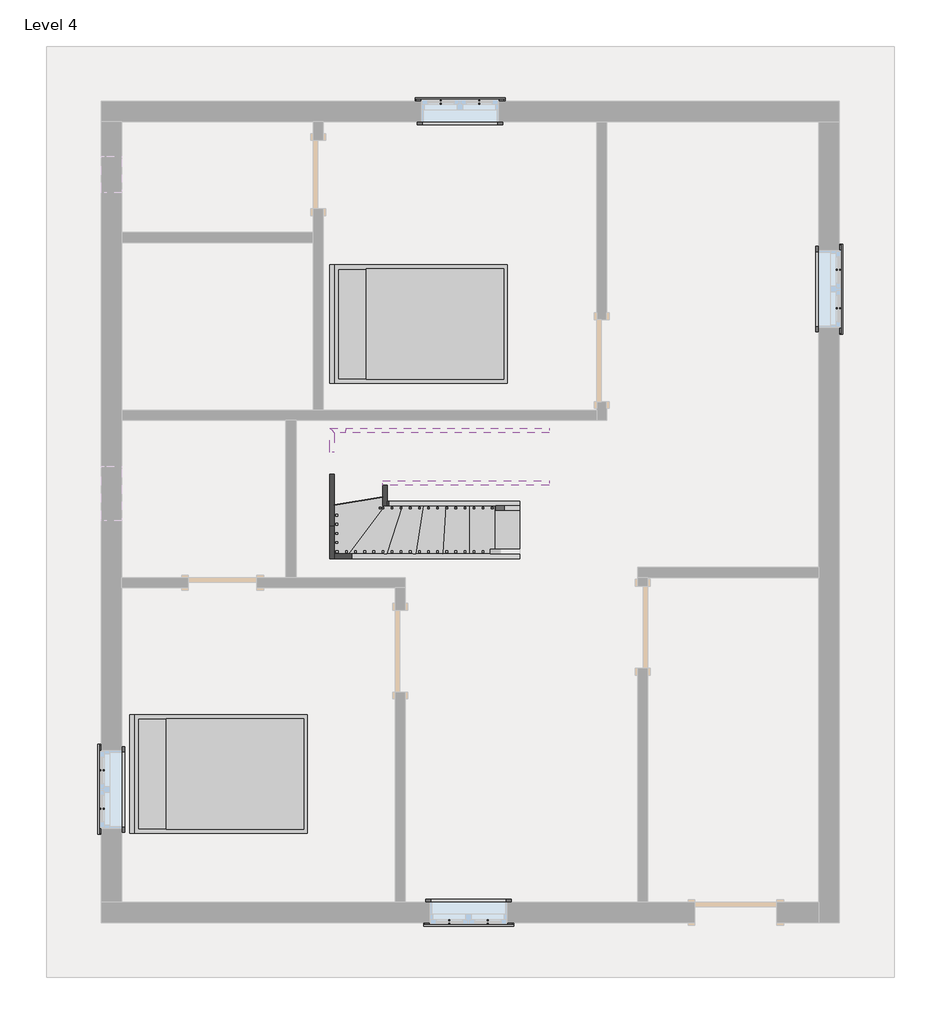
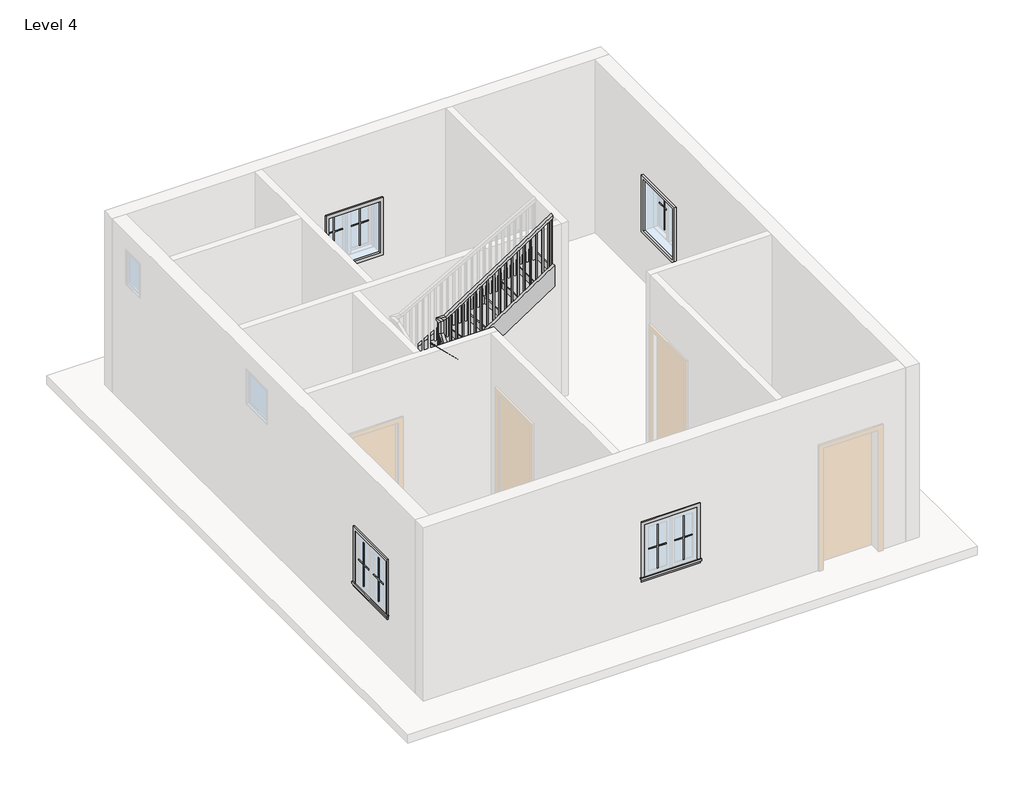
# One storey, part 2 of 2: 16 proxies, 9 members, 2 furniture elements, 1 railing, 1 stair flight.
"""IFC4 building model written with IfcOpenShell, lengths in millimetres."""

from ifc_helpers import new_model, si_unit, frame, origin, place, context, project, spatial, polyline, outline, extrude, faceted_brep, transform, mapped, element, save
from components import muntin_pattern_2x2_muntin_pattern_2x2_b3fe6957, muntin_pattern_2x2_muntin_pattern_2x2_3e0ecaf2, trim_window_exterior_flat_with_sill_41619996, trim_window_interior_flat_picture_frame_51c85655, bed_17739_bed_17739_15c61121, stair_flight_033e9654

model = new_model("IFC4")

# Units and contexts
model_context = context("Model", 3, world=origin())
ifc_project = project(units=[si_unit("LENGTHUNIT", "METRE", prefix="MILLI")], contexts=[model_context])

# Site, building, storey
site = spatial("IfcSite", under=ifc_project)
building = spatial("IfcBuilding", under=site)
storey = spatial("IfcBuildingStorey", under=building, Name="Level 4", Elevation=6400.8)

# Proxies
placement = place(None, origin())
muntin_pattern_2x2_muntin_pattern_2x2_shape = muntin_pattern_2x2_muntin_pattern_2x2_b3fe6957(model_context)
element("IfcBuildingElementProxy", 1, Name="Muntin Pattern_2x2 : Muntin Pattern_2x2", ObjectType="Muntin Pattern_2x2 : Muntin Pattern_2x2", at=placement, inside=storey, context=model_context, shape_type="MappedRepresentation", body=[
    mapped(muntin_pattern_2x2_muntin_pattern_2x2_shape, transform((-1143.3273498, 4766.5933073, 7385.05), x_axis=(1.0, 0.0, 0.0), y_axis=(0.0, 1.0, 0.0), z_axis=(0.0, 0.0, 1.0))),
])
element("IfcBuildingElementProxy", 2, Name="Muntin Pattern_2x2 : Muntin Pattern_2x2", ObjectType="Muntin Pattern_2x2 : Muntin Pattern_2x2", at=placement, inside=storey, context=model_context, shape_type="MappedRepresentation", body=[
    mapped(muntin_pattern_2x2_muntin_pattern_2x2_shape, transform((3290.5601502, 2894.9308073, 7385.05), x_axis=(0.0, -1.0, 0.0), y_axis=(1.0, 0.0, 0.0), z_axis=(0.0, 0.0, 1.0))),
])
element("IfcBuildingElementProxy", 3, Name="Muntin Pattern_2x2 : Muntin Pattern_2x2", ObjectType="Muntin Pattern_2x2 : Muntin Pattern_2x2", at=placement, inside=storey, context=model_context, shape_type="MappedRepresentation", body=[
    mapped(muntin_pattern_2x2_muntin_pattern_2x2_shape, transform((-619.4523498, -4374.2316927, 7385.05), x_axis=(-1.0, 0.0, 0.0), y_axis=(0.0, -1.0, 0.0), z_axis=(0.0, 0.0, 1.0))),
])
element("IfcBuildingElementProxy", 4, Name="Muntin Pattern_2x2 : Muntin Pattern_2x2", ObjectType="Muntin Pattern_2x2 : Muntin Pattern_2x2", at=placement, inside=storey, context=model_context, shape_type="MappedRepresentation", body=[
    mapped(muntin_pattern_2x2_muntin_pattern_2x2_shape, transform((-4919.9898498, -3112.1691927, 7385.05), x_axis=(0.0, 1.0, 0.0), y_axis=(-1.0, 0.0, 0.0), z_axis=(0.0, 0.0, 1.0))),
])
muntin_pattern_2x2_muntin_pattern_2x2_2_shape = muntin_pattern_2x2_muntin_pattern_2x2_3e0ecaf2(model_context)
element("IfcBuildingElementProxy", 5, Name="Muntin Pattern_2x2 : Muntin Pattern_2x2", ObjectType="Muntin Pattern_2x2 : Muntin Pattern_2x2", at=placement, inside=storey, context=model_context, shape_type="MappedRepresentation", body=[
    mapped(muntin_pattern_2x2_muntin_pattern_2x2_2_shape, transform((-714.7023498, 4766.5933073, 7385.05), x_axis=(-1.0, 0.0, 0.0), y_axis=(0.0, -1.0, 0.0), z_axis=(0.0, 0.0, 1.0))),
])
element("IfcBuildingElementProxy", 6, Name="Muntin Pattern_2x2 : Muntin Pattern_2x2", ObjectType="Muntin Pattern_2x2 : Muntin Pattern_2x2", at=placement, inside=storey, context=model_context, shape_type="MappedRepresentation", body=[
    mapped(muntin_pattern_2x2_muntin_pattern_2x2_2_shape, transform((3290.5601502, 2466.3058073, 7385.05), x_axis=(0.0, 1.0, 0.0), y_axis=(-1.0, 0.0, 0.0), z_axis=(0.0, 0.0, 1.0))),
])
element("IfcBuildingElementProxy", 7, Name="Muntin Pattern_2x2 : Muntin Pattern_2x2", ObjectType="Muntin Pattern_2x2 : Muntin Pattern_2x2", at=placement, inside=storey, context=model_context, shape_type="MappedRepresentation", body=[
    mapped(muntin_pattern_2x2_muntin_pattern_2x2_2_shape, transform((-1048.0773498, -4374.2316927, 7385.05), x_axis=(1.0, 0.0, 0.0), y_axis=(0.0, 1.0, 0.0), z_axis=(0.0, 0.0, 1.0))),
])
element("IfcBuildingElementProxy", 8, Name="Muntin Pattern_2x2 : Muntin Pattern_2x2", ObjectType="Muntin Pattern_2x2 : Muntin Pattern_2x2", at=placement, inside=storey, context=model_context, shape_type="MappedRepresentation", body=[
    mapped(muntin_pattern_2x2_muntin_pattern_2x2_2_shape, transform((-4919.9898498, -2683.5441927, 7385.05), x_axis=(0.0, -1.0, 0.0), y_axis=(1.0, 0.0, 0.0), z_axis=(0.0, 0.0, 1.0))),
])
trim_window_exterior_flat_with_sill_shape = trim_window_exterior_flat_with_sill_41619996(model_context)
element("IfcBuildingElementProxy", 9, Name="Trim-Window-Exterior-Flat : with Sill", ObjectType="Trim-Window-Exterior-Flat : with Sill", at=placement, inside=storey, context=model_context, shape_type="MappedRepresentation", body=[
    mapped(trim_window_exterior_flat_with_sill_shape, transform((-929.0148498, 4776.1183073, 8229.6), x_axis=(-1.0, 0.0, 0.0), y_axis=(0.0, 0.0, 1.0), z_axis=(0.0, 1.0, 0.0))),
])
element("IfcBuildingElementProxy", 10, Name="Trim-Window-Exterior-Flat : with Sill", ObjectType="Trim-Window-Exterior-Flat : with Sill", at=placement, inside=storey, context=model_context, shape_type="MappedRepresentation", body=[
    mapped(trim_window_exterior_flat_with_sill_shape, transform((3300.0851502, 2680.6183073, 8229.6), x_axis=(0.0, 1.0, 0.0), y_axis=(0.0, 0.0, 1.0), z_axis=(1.0, 0.0, 0.0))),
])
element("IfcBuildingElementProxy", 11, Name="Trim-Window-Exterior-Flat : with Sill", ObjectType="Trim-Window-Exterior-Flat : with Sill", at=placement, inside=storey, context=model_context, shape_type="MappedRepresentation", body=[
    mapped(trim_window_exterior_flat_with_sill_shape, transform((-833.7648498, -4383.7566927, 8229.6), x_axis=(1.0, 0.0, 0.0), y_axis=(0.0, 0.0, 1.0), z_axis=(0.0, -1.0, 0.0))),
])
element("IfcBuildingElementProxy", 12, Name="Trim-Window-Exterior-Flat : with Sill", ObjectType="Trim-Window-Exterior-Flat : with Sill", at=placement, inside=storey, context=model_context, shape_type="MappedRepresentation", body=[
    mapped(trim_window_exterior_flat_with_sill_shape, transform((-4929.5148498, -2897.8566927, 8229.6), x_axis=(0.0, -1.0, 0.0), y_axis=(0.0, 0.0, 1.0), z_axis=(-1.0, 0.0, 0.0))),
])
trim_window_interior_flat_picture_frame_shape = trim_window_interior_flat_picture_frame_51c85655(model_context)
element("IfcBuildingElementProxy", 13, Name="Trim-Window-Interior-Flat : Picture Frame", ObjectType="Trim-Window-Interior-Flat : Picture Frame", at=placement, inside=storey, context=model_context, shape_type="MappedRepresentation", body=[
    mapped(trim_window_interior_flat_picture_frame_shape, transform((-929.0148498, 4547.5183073, 8229.6), x_axis=(1.0, 0.0, 0.0), y_axis=(0.0, 0.0, 1.0), z_axis=(0.0, -1.0, 0.0))),
])
element("IfcBuildingElementProxy", 14, Name="Trim-Window-Interior-Flat : Picture Frame", ObjectType="Trim-Window-Interior-Flat : Picture Frame", at=placement, inside=storey, context=model_context, shape_type="MappedRepresentation", body=[
    mapped(trim_window_interior_flat_picture_frame_shape, transform((3071.4851502, 2680.6183073, 8229.6), x_axis=(0.0, -1.0, 0.0), y_axis=(0.0, 0.0, 1.0), z_axis=(-1.0, 0.0, 0.0))),
])
element("IfcBuildingElementProxy", 15, Name="Trim-Window-Interior-Flat : Picture Frame", ObjectType="Trim-Window-Interior-Flat : Picture Frame", at=placement, inside=storey, context=model_context, shape_type="MappedRepresentation", body=[
    mapped(trim_window_interior_flat_picture_frame_shape, transform((-833.7648498, -4155.1566927, 8229.6), x_axis=(-1.0, 0.0, 0.0), y_axis=(0.0, 0.0, 1.0), z_axis=(0.0, 1.0, 0.0))),
])
element("IfcBuildingElementProxy", 16, Name="Trim-Window-Interior-Flat : Picture Frame", ObjectType="Trim-Window-Interior-Flat : Picture Frame", at=placement, inside=storey, context=model_context, shape_type="MappedRepresentation", body=[
    mapped(trim_window_interior_flat_picture_frame_shape, transform((-4700.9148498, -2897.8566927, 8229.6), x_axis=(0.0, 1.0, 0.0), y_axis=(0.0, 0.0, 1.0), z_axis=(1.0, 0.0, 0.0))),
])

# Furniture
bed_17739_bed_17739_shape = bed_17739_bed_17739_15c61121(model_context)
element("IfcFurniture", 17, ObjectType="Bed_17739 : Bed_17739", at=placement, inside=storey, context=model_context, shape_type="MappedRepresentation", body=[
    mapped(bed_17739_bed_17739_shape, transform((-3596.0148498, -2726.4066927, 6400.8), x_axis=(0.0, 1.0, 0.0), y_axis=(-1.0, 0.0, 0.0), z_axis=(0.0, 0.0, 1.0))),
])
element("IfcFurniture", 18, ObjectType="Bed_17739 : Bed_17739", at=placement, inside=storey, context=model_context, shape_type="MappedRepresentation", body=[
    mapped(bed_17739_bed_17739_shape, transform((-1367.1648498, 2290.0933073, 6400.8), x_axis=(0.0, 1.0, 0.0), y_axis=(-1.0, 0.0, 0.0), z_axis=(0.0, 0.0, 1.0))),
])

# Members
element("IfcMember", 19, ObjectType="Stringer - 2\" Width", at=placement, inside=storey, context=model_context, shape_type="SweptSolid", body=[
    extrude(outline(polyline([(6400.8, -264.8831579), (6629.2652135, -264.8831579), (7705.0576628, -2328.8610857), (7361.3393024, -2328.8610857), (6400.8, -486.0038318), (6400.8, -264.8831579)])), frame((0.0, -322.6029286, 0.0), z_axis=(0.0, 1.0, 0.0), x_axis=(0.0, 0.0, 1.0)), (0.0, 0.0, 1.0), 50.8),
])
element("IfcMember", 20, ObjectType="Stringer - 2\" Width", at=placement, inside=storey, context=model_context, shape_type="SweptSolid", body=[
    extrude(outline(polyline([(-2328.8610857, -322.6029286), (-2379.6610857, -322.6029286), (-2379.6610857, 39.7116887), (-2328.8610857, 39.7116887), (-2328.8610857, -322.6029286)])), frame((0.0, 0.0, 7361.3393024), z_axis=(0.0, 0.0, 1.0), x_axis=(1.0, 0.0, 0.0)), (0.0, 0.0, 1.0), 343.7183604),
])
element("IfcMember", 21, ObjectType="Stringer - 2\" Width", at=placement, inside=storey, context=model_context, shape_type="SweptSolid", body=[
    extrude(outline(polyline([(39.7116887, 7361.3393024), (39.7116887, 7705.0576628), (861.172384, 8044.8948766), (861.172384, 7701.1765162), (39.7116887, 7361.3393024)])), frame((-2379.6610857, 0.0, 0.0), z_axis=(1.0, 0.0, 0.0), x_axis=(0.0, 1.0, 0.0)), (0.0, 0.0, 1.0), 50.8),
])
element("IfcMember", 22, ObjectType="Stringer - 2\" Width", at=placement, inside=storey, context=model_context, shape_type="SweptSolid", body=[
    extrude(outline(polyline([(-2328.8610857, 861.172384), (-2379.6610857, 861.172384), (-2379.6610857, 1130.8895433), (-2328.8610857, 1080.0895433), (-2328.8610857, 861.172384)])), frame((0.0, 0.0, 7707.4790002), z_axis=(0.0, 0.0, 1.0), x_axis=(1.0, 0.0, 0.0)), (0.0, 0.0, 1.0), 329.8531189),
])
element("IfcMember", 23, ObjectType="Stringer - 2\" Width", at=placement, inside=storey, context=model_context, shape_type="SweptSolid", body=[
    extrude(outline(polyline([(-2328.8610857, 1080.0895433), (-2379.6610857, 1130.8895433), (-2203.9193363, 1130.8895433), (-2203.9193363, 1080.0895433), (-2328.8610857, 1080.0895433)])), frame((0.0, 0.0, 7707.4790002), z_axis=(0.0, 0.0, 1.0), x_axis=(1.0, 0.0, 0.0)), (0.0, 0.0, 1.0), 329.8531189),
])
element("IfcMember", 24, ObjectType="Stringer - 2\" Width", at=placement, inside=storey, context=model_context, shape_type="SweptSolid", body=[
    extrude(outline(polyline([(6400.8, -264.8831579), (6597.7581828, -264.8831579), (7617.2545254, -1741.8148498), (7246.8897368, -1741.8148498), (6400.8, -516.0951544), (6400.8, -264.8831579)])), frame((0.0, 264.4433073, 0.0), z_axis=(0.0, 1.0, 0.0), x_axis=(0.0, 0.0, 1.0)), (0.0, 0.0, 1.0), 50.8),
])
element("IfcMember", 25, ObjectType="Stringer - 2\" Width", at=placement, inside=storey, context=model_context, shape_type="SweptSolid", body=[
    extrude(outline(polyline([(264.4433073, 7326.5590756), (264.4433073, 7785.758282), (493.0433073, 8043.3490234), (493.0433073, 7584.149817), (264.4433073, 7326.5590756)])), frame((-1792.6148498, 0.0, 0.0), z_axis=(1.0, 0.0, 0.0), x_axis=(0.0, 1.0, 0.0)), (0.0, 0.0, 1.0), 50.8),
])
element("IfcMember", 26, ObjectType="Stringer - 2\" Width", at=placement, inside=storey, context=model_context, shape_type="SweptSolid", body=[
    extrude(outline(polyline([(8116.4438732, -1792.6148498), (7751.1121415, -1792.6148498), (8977.5313098, 63.4034409), (9342.8630415, 63.4034409), (8116.4438732, -1792.6148498)])), frame((0.0, 493.0433073, 0.0), z_axis=(0.0, 1.0, 0.0), x_axis=(0.0, 0.0, 1.0)), (0.0, 0.0, 1.0), 50.8),
])
element("IfcMember", 27, ObjectType="Stringer - 2\" Width", at=placement, inside=storey, context=model_context, shape_type="SweptSolid", body=[
    extrude(outline(polyline([(8037.332119, -2203.9193363), (7707.4790002, -2203.9193363), (8962.842957, 63.4034409), (9292.6960758, 63.4034409), (8037.332119, -2203.9193363)])), frame((0.0, 1080.0895433, 0.0), z_axis=(0.0, 1.0, 0.0), x_axis=(0.0, 0.0, 1.0)), (0.0, 0.0, 1.0), 50.8),
])

# Railing
element("IfcRailing", 28, ObjectType="Handrail - Rectangular", at=placement, inside=storey, context=model_context, shape_type="SolidModel", body=[
    faceted_brep([(-264.8831579, 213.6433073, 7484.5333333), (-264.8831579, 213.6433073, 7423.2533076), (-264.8831579, 264.4433073, 7423.2533076), (-264.8831579, 264.4433073, 7484.5333333), (-1716.4148498, 213.6433073, 8463.8160626), (-1767.2148498, 213.6433073, 8436.8084974), (-1767.2148498, 264.4433073, 8436.8084974), (-1716.4148498, 264.4433073, 8463.8160626), (-1716.4148498, 213.6433073, 8678.3989826), (-1767.2148498, 213.6433073, 8627.5989826), (-1767.2148498, 264.4433073, 8627.5989826), (-1716.4148498, 264.4433073, 8678.3989826), (-1843.4148498, 213.6433073, 8678.3989826), (-1843.4148498, 213.6433073, 8627.5989826), (-1792.6148498, 264.4433073, 8627.5989826), (-1792.6148498, 264.4433073, 8678.3989826), (-1843.4148498, 340.6433073, 8678.3989826), (-1843.4148498, 363.4803462, 8627.5989826), (-1792.6148498, 363.4803462, 8627.5989826), (-1792.6148498, 340.6433073, 8678.3989826), (-1843.4148498, 467.6433073, 8821.50495), (-1843.4148498, 518.4433073, 8802.2141359), (-1792.6148498, 518.4433073, 8802.2141359), (-1792.6148498, 467.6433073, 8821.50495), (-1843.4148498, 467.6433073, 9032.774751), (-1843.4148498, 518.4433073, 8981.974751), (-1792.6148498, 518.4433073, 8981.974751), (-1792.6148498, 467.6433073, 9032.774751), (-1843.4148498, 594.6433073, 9032.774751), (-1843.4148498, 594.6433073, 8981.974751), (-1792.6148498, 543.8433073, 8981.974751), (-1792.6148498, 543.8433073, 9032.774751), (-1716.4148498, 594.6433073, 9032.774751), (-1701.3097842, 594.6433073, 8981.974751), (-1701.3097842, 543.8433073, 8981.974751), (-1716.4148498, 543.8433073, 9032.774751), (63.4034409, 594.6433073, 10193.8666667), (63.4034409, 543.8433073, 10193.8666667), (63.4034409, 543.8433073, 10133.2126442), (63.4034409, 594.6433073, 10133.2126442)], [[[0, 1, 2, 3]], [[1, 0, 4, 5]], [[2, 1, 5, 6]], [[3, 2, 6, 7]], [[0, 3, 7, 4]], [[5, 4, 8, 9]], [[6, 5, 9, 10]], [[7, 6, 10, 11]], [[4, 7, 11, 8]], [[9, 8, 12, 13]], [[10, 9, 13, 14]], [[11, 10, 14, 15]], [[8, 11, 15, 12]], [[13, 12, 16, 17]], [[14, 13, 17, 18]], [[15, 14, 18, 19]], [[12, 15, 19, 16]], [[17, 16, 20, 21]], [[18, 17, 21, 22]], [[19, 18, 22, 23]], [[16, 19, 23, 20]], [[21, 20, 24, 25]], [[22, 21, 25, 26]], [[23, 22, 26, 27]], [[20, 23, 27, 24]], [[25, 24, 28, 29]], [[26, 25, 29, 30]], [[27, 26, 30, 31]], [[24, 27, 31, 28]], [[29, 28, 32, 33]], [[30, 29, 33, 34]], [[31, 30, 34, 35]], [[28, 31, 35, 32]], [[36, 37, 38, 39]], [[33, 32, 36, 39]], [[34, 33, 39, 38]], [[35, 34, 38, 37]], [[32, 35, 37, 36]]]),
    extrude(outline(polyline([(10105.1000713, 20.3101502), (10092.67251, 1.2601502), (9110.1333333, 1.2601502), (9110.1333333, 20.3101502), (10105.1000713, 20.3101502)])), frame((0.0, 559.7183073, 0.0), z_axis=(0.0, 1.0, 0.0), x_axis=(0.0, 0.0, 1.0)), (0.0, 0.0, 1.0), 19.05),
    extrude(outline(polyline([(10038.8197441, -81.2898498), (10026.3921828, -100.3398498), (9110.1333333, -100.3398498), (9110.1333333, -81.2898498), (10038.8197441, -81.2898498)])), frame((0.0, 559.7183073, 0.0), z_axis=(0.0, 1.0, 0.0), x_axis=(0.0, 0.0, 1.0)), (0.0, 0.0, 1.0), 19.05),
    extrude(outline(polyline([(9972.539417, -182.8898498), (9960.1118556, -201.9398498), (9110.1333333, -201.9398498), (9110.1333333, -182.8898498), (9972.539417, -182.8898498)])), frame((0.0, 559.7183073, 0.0), z_axis=(0.0, 1.0, 0.0), x_axis=(0.0, 0.0, 1.0)), (0.0, 0.0, 1.0), 19.05),
    extrude(outline(polyline([(9906.2590898, -284.4898498), (9893.8315284, -303.5398498), (8940.8, -303.5398498), (8940.8, -284.4898498), (9906.2590898, -284.4898498)])), frame((0.0, 559.7183073, 0.0), z_axis=(0.0, 1.0, 0.0), x_axis=(0.0, 0.0, 1.0)), (0.0, 0.0, 1.0), 19.05),
    extrude(outline(polyline([(9839.9787626, -386.0898498), (9827.5512012, -405.1398498), (8940.8, -405.1398498), (8940.8, -386.0898498), (9839.9787626, -386.0898498)])), frame((0.0, 559.7183073, 0.0), z_axis=(0.0, 1.0, 0.0), x_axis=(0.0, 0.0, 1.0)), (0.0, 0.0, 1.0), 19.05),
    extrude(outline(polyline([(9773.6984354, -487.6898498), (9761.2708741, -506.7398498), (8771.4666667, -506.7398498), (8771.4666667, -487.6898498), (9773.6984354, -487.6898498)])), frame((0.0, 559.7183073, 0.0), z_axis=(0.0, 1.0, 0.0), x_axis=(0.0, 0.0, 1.0)), (0.0, 0.0, 1.0), 19.05),
    extrude(outline(polyline([(9707.4181082, -589.2898498), (9694.9905469, -608.3398498), (8771.4666667, -608.3398498), (8771.4666667, -589.2898498), (9707.4181082, -589.2898498)])), frame((0.0, 559.7183073, 0.0), z_axis=(0.0, 1.0, 0.0), x_axis=(0.0, 0.0, 1.0)), (0.0, 0.0, 1.0), 19.05),
    extrude(outline(polyline([(9641.1377811, -690.8898498), (9628.7102197, -709.9398498), (8771.4666667, -709.9398498), (8771.4666667, -690.8898498), (9641.1377811, -690.8898498)])), frame((0.0, 559.7183073, 0.0), z_axis=(0.0, 1.0, 0.0), x_axis=(0.0, 0.0, 1.0)), (0.0, 0.0, 1.0), 19.05),
    extrude(outline(polyline([(9574.8574539, -792.4898498), (9562.4298925, -811.5398498), (8602.1333333, -811.5398498), (8602.1333333, -792.4898498), (9574.8574539, -792.4898498)])), frame((0.0, 559.7183073, 0.0), z_axis=(0.0, 1.0, 0.0), x_axis=(0.0, 0.0, 1.0)), (0.0, 0.0, 1.0), 19.05),
    extrude(outline(polyline([(9508.5771267, -894.0898498), (9496.1495653, -913.1398498), (8602.1333333, -913.1398498), (8602.1333333, -894.0898498), (9508.5771267, -894.0898498)])), frame((0.0, 559.7183073, 0.0), z_axis=(0.0, 1.0, 0.0), x_axis=(0.0, 0.0, 1.0)), (0.0, 0.0, 1.0), 19.05),
    extrude(outline(polyline([(9442.2967995, -995.6898498), (9429.8692382, -1014.7398498), (8602.1333333, -1014.7398498), (8602.1333333, -995.6898498), (9442.2967995, -995.6898498)])), frame((0.0, 559.7183073, 0.0), z_axis=(0.0, 1.0, 0.0), x_axis=(0.0, 0.0, 1.0)), (0.0, 0.0, 1.0), 19.05),
    extrude(outline(polyline([(9376.0164723, -1097.2898498), (9363.588911, -1116.3398498), (8432.8, -1116.3398498), (8432.8, -1097.2898498), (9376.0164723, -1097.2898498)])), frame((0.0, 559.7183073, 0.0), z_axis=(0.0, 1.0, 0.0), x_axis=(0.0, 0.0, 1.0)), (0.0, 0.0, 1.0), 19.05),
    extrude(outline(polyline([(9309.7361451, -1198.8898498), (9297.3085838, -1217.9398498), (8432.8, -1217.9398498), (8432.8, -1198.8898498), (9309.7361451, -1198.8898498)])), frame((0.0, 559.7183073, 0.0), z_axis=(0.0, 1.0, 0.0), x_axis=(0.0, 0.0, 1.0)), (0.0, 0.0, 1.0), 19.05),
    extrude(outline(polyline([(9243.455818, -1300.4898498), (9231.0282566, -1319.5398498), (8263.4666667, -1319.5398498), (8263.4666667, -1300.4898498), (9243.455818, -1300.4898498)])), frame((0.0, 559.7183073, 0.0), z_axis=(0.0, 1.0, 0.0), x_axis=(0.0, 0.0, 1.0)), (0.0, 0.0, 1.0), 19.05),
    extrude(outline(polyline([(9177.1754908, -1402.0898498), (9164.7479294, -1421.1398498), (8263.4666667, -1421.1398498), (8263.4666667, -1402.0898498), (9177.1754908, -1402.0898498)])), frame((0.0, 559.7183073, 0.0), z_axis=(0.0, 1.0, 0.0), x_axis=(0.0, 0.0, 1.0)), (0.0, 0.0, 1.0), 19.05),
    extrude(outline(polyline([(9110.8951636, -1503.6898498), (9098.4676023, -1522.7398498), (8263.4666667, -1522.7398498), (8263.4666667, -1503.6898498), (9110.8951636, -1503.6898498)])), frame((0.0, 559.7183073, 0.0), z_axis=(0.0, 1.0, 0.0), x_axis=(0.0, 0.0, 1.0)), (0.0, 0.0, 1.0), 19.05),
    extrude(outline(polyline([(9044.6148364, -1605.2898498), (9032.1872751, -1624.3398498), (8094.1333333, -1624.3398498), (8094.1333333, -1605.2898498), (9044.6148364, -1605.2898498)])), frame((0.0, 559.7183073, 0.0), z_axis=(0.0, 1.0, 0.0), x_axis=(0.0, 0.0, 1.0)), (0.0, 0.0, 1.0), 19.05),
    extrude(outline(polyline([(8978.3345092, -1706.8898498), (8965.9069479, -1725.9398498), (8094.1333333, -1725.9398498), (8094.1333333, -1706.8898498), (8978.3345092, -1706.8898498)])), frame((0.0, 559.7183073, 0.0), z_axis=(0.0, 1.0, 0.0), x_axis=(0.0, 0.0, 1.0)), (0.0, 0.0, 1.0), 19.05),
    extrude(outline(polyline([(-1808.4898498, 534.3183073), (-1827.5398498, 534.3183073), (-1827.5398498, 553.3683073), (-1808.4898498, 553.3683073), (-1808.4898498, 534.3183073)])), frame((0.0, 0.0, 7924.8), z_axis=(0.0, 0.0, 1.0), x_axis=(1.0, 0.0, 0.0)), (0.0, 0.0, 1.0), 1057.174751),
    extrude(outline(polyline([(432.7183073, 8705.6176079), (451.7683073, 8727.083503), (451.7683073, 7755.4666667), (432.7183073, 7755.4666667), (432.7183073, 8705.6176079)])), frame((-1827.5398498, 0.0, 0.0), z_axis=(1.0, 0.0, 0.0), x_axis=(0.0, 1.0, 0.0)), (0.0, 0.0, 1.0), 19.05),
    extrude(outline(polyline([(331.1183073, 8591.132834), (350.1683073, 8612.5987291), (350.1683073, 7755.4666667), (331.1183073, 7755.4666667), (331.1183073, 8591.132834)])), frame((-1827.5398498, 0.0, 0.0), z_axis=(1.0, 0.0, 0.0), x_axis=(0.0, 1.0, 0.0)), (0.0, 0.0, 1.0), 19.05),
    extrude(outline(polyline([(-1779.3581579, 248.5683073), (-1779.3581579, 229.5183073), (-1798.4081579, 229.5183073), (-1798.4081579, 248.5683073), (-1779.3581579, 248.5683073)])), frame((0.0, 0.0, 7416.8), z_axis=(0.0, 0.0, 1.0), x_axis=(1.0, 0.0, 0.0)), (0.0, 0.0, 1.0), 1210.7989826),
    extrude(outline(polyline([(8376.4561166, -1677.7581579), (8389.3082893, -1696.8081579), (7416.8, -1696.8081579), (7416.8, -1677.7581579), (8376.4561166, -1677.7581579)])), frame((0.0, 229.5183073, 0.0), z_axis=(0.0, 1.0, 0.0), x_axis=(0.0, 0.0, 1.0)), (0.0, 0.0, 1.0), 19.05),
    extrude(outline(polyline([(8307.9111955, -1576.1581579), (8320.7633682, -1595.2081579), (7416.8, -1595.2081579), (7416.8, -1576.1581579), (8307.9111955, -1576.1581579)])), frame((0.0, 229.5183073, 0.0), z_axis=(0.0, 1.0, 0.0), x_axis=(0.0, 0.0, 1.0)), (0.0, 0.0, 1.0), 19.05),
    extrude(outline(polyline([(8239.3662744, -1474.5581579), (8252.2184472, -1493.6081579), (7247.4666667, -1493.6081579), (7247.4666667, -1474.5581579), (8239.3662744, -1474.5581579)])), frame((0.0, 229.5183073, 0.0), z_axis=(0.0, 1.0, 0.0), x_axis=(0.0, 0.0, 1.0)), (0.0, 0.0, 1.0), 19.05),
    extrude(outline(polyline([(8170.8213533, -1372.9581579), (8183.6735261, -1392.0081579), (7247.4666667, -1392.0081579), (7247.4666667, -1372.9581579), (8170.8213533, -1372.9581579)])), frame((0.0, 229.5183073, 0.0), z_axis=(0.0, 1.0, 0.0), x_axis=(0.0, 0.0, 1.0)), (0.0, 0.0, 1.0), 19.05),
    extrude(outline(polyline([(8102.2764322, -1271.3581579), (8115.128605, -1290.4081579), (7078.1333333, -1290.4081579), (7078.1333333, -1271.3581579), (8102.2764322, -1271.3581579)])), frame((0.0, 229.5183073, 0.0), z_axis=(0.0, 1.0, 0.0), x_axis=(0.0, 0.0, 1.0)), (0.0, 0.0, 1.0), 19.05),
    extrude(outline(polyline([(8033.7315111, -1169.7581579), (8046.5836839, -1188.8081579), (7078.1333333, -1188.8081579), (7078.1333333, -1169.7581579), (8033.7315111, -1169.7581579)])), frame((0.0, 229.5183073, 0.0), z_axis=(0.0, 1.0, 0.0), x_axis=(0.0, 0.0, 1.0)), (0.0, 0.0, 1.0), 19.05),
    extrude(outline(polyline([(7965.18659, -1068.1581579), (7978.0387628, -1087.2081579), (6908.8, -1087.2081579), (6908.8, -1068.1581579), (7965.18659, -1068.1581579)])), frame((0.0, 229.5183073, 0.0), z_axis=(0.0, 1.0, 0.0), x_axis=(0.0, 0.0, 1.0)), (0.0, 0.0, 1.0), 19.05),
    extrude(outline(polyline([(7896.641669, -966.5581579), (7909.4938417, -985.6081579), (6908.8, -985.6081579), (6908.8, -966.5581579), (7896.641669, -966.5581579)])), frame((0.0, 229.5183073, 0.0), z_axis=(0.0, 1.0, 0.0), x_axis=(0.0, 0.0, 1.0)), (0.0, 0.0, 1.0), 19.05),
    extrude(outline(polyline([(7828.0967479, -864.9581579), (7840.9489206, -884.0081579), (6908.8, -884.0081579), (6908.8, -864.9581579), (7828.0967479, -864.9581579)])), frame((0.0, 229.5183073, 0.0), z_axis=(0.0, 1.0, 0.0), x_axis=(0.0, 0.0, 1.0)), (0.0, 0.0, 1.0), 19.05),
    extrude(outline(polyline([(7759.5518268, -763.3581579), (7772.4039995, -782.4081579), (6739.4666667, -782.4081579), (6739.4666667, -763.3581579), (7759.5518268, -763.3581579)])), frame((0.0, 229.5183073, 0.0), z_axis=(0.0, 1.0, 0.0), x_axis=(0.0, 0.0, 1.0)), (0.0, 0.0, 1.0), 19.05),
    extrude(outline(polyline([(7691.0069057, -661.7581579), (7703.8590784, -680.8081579), (6739.4666667, -680.8081579), (6739.4666667, -661.7581579), (7691.0069057, -661.7581579)])), frame((0.0, 229.5183073, 0.0), z_axis=(0.0, 1.0, 0.0), x_axis=(0.0, 0.0, 1.0)), (0.0, 0.0, 1.0), 19.05),
    extrude(outline(polyline([(7622.4619846, -560.1581579), (7635.3141573, -579.2081579), (6739.4666667, -579.2081579), (6739.4666667, -560.1581579), (7622.4619846, -560.1581579)])), frame((0.0, 229.5183073, 0.0), z_axis=(0.0, 1.0, 0.0), x_axis=(0.0, 0.0, 1.0)), (0.0, 0.0, 1.0), 19.05),
    extrude(outline(polyline([(7553.9170635, -458.5581579), (7566.7692362, -477.6081579), (6570.1333333, -477.6081579), (6570.1333333, -458.5581579), (7553.9170635, -458.5581579)])), frame((0.0, 229.5183073, 0.0), z_axis=(0.0, 1.0, 0.0), x_axis=(0.0, 0.0, 1.0)), (0.0, 0.0, 1.0), 19.05),
    extrude(outline(polyline([(7485.3721424, -356.9581579), (7498.2243151, -376.0081579), (6570.1333333, -376.0081579), (6570.1333333, -356.9581579), (7485.3721424, -356.9581579)])), frame((0.0, 229.5183073, 0.0), z_axis=(0.0, 1.0, 0.0), x_axis=(0.0, 0.0, 1.0)), (0.0, 0.0, 1.0), 19.05),
    extrude(outline(polyline([(-1808.4898498, 559.7183073), (-1827.5398498, 559.7183073), (-1827.5398498, 578.7683073), (-1808.4898498, 578.7683073), (-1808.4898498, 559.7183073)])), frame((0.0, 0.0, 7924.8), z_axis=(0.0, 0.0, 1.0), x_axis=(1.0, 0.0, 0.0)), (0.0, 0.0, 1.0), 1057.174751),
    extrude(outline(polyline([(-1808.4898498, 248.5683073), (-1808.4898498, 229.5183073), (-1827.5398498, 229.5183073), (-1827.5398498, 248.5683073), (-1808.4898498, 248.5683073)])), frame((0.0, 0.0, 7586.1333333), z_axis=(0.0, 0.0, 1.0), x_axis=(1.0, 0.0, 0.0)), (0.0, 0.0, 1.0), 1041.4656493),
    extrude(outline(polyline([(10133.2126442, 63.4034409), (10120.7850828, 44.3534409), (9110.1333333, 44.3534409), (9110.1333333, 63.4034409), (10133.2126442, 63.4034409)])), frame((0.0, 559.7183073, 0.0), z_axis=(0.0, 1.0, 0.0), x_axis=(0.0, 0.0, 1.0)), (0.0, 0.0, 1.0), 19.05),
    extrude(outline(polyline([(7423.2533076, -264.8831579), (7436.1054803, -283.9331579), (6570.1333333, -283.9331579), (6570.1333333, -264.8831579), (7423.2533076, -264.8831579)])), frame((0.0, 229.5183073, 0.0), z_axis=(0.0, 1.0, 0.0), x_axis=(0.0, 0.0, 1.0)), (0.0, 0.0, 1.0), 19.05),
])

# Stair flight
stair_flight_shape = stair_flight_033e9654(model_context)
element("IfcStairFlight", 29, ObjectType="2\" Tread 1\" Nosing 1/4\" Riser", at=placement, inside=storey, context=model_context, shape_type="MappedRepresentation", body=[
    mapped(stair_flight_shape, transform((0.0, 0.0, 0.0), x_axis=(1.0, 0.0, 0.0), y_axis=(0.0, 1.0, 0.0), z_axis=(0.0, 0.0, 1.0))),
])

save(model, "model.ifc")

# Revit data of these elements
# Type "Muntin Pattern_2x2 : Muntin Pattern_2x2"
#   Width [instance default] = 4' - 0"
#   Thickness = 0' - 0 1/2"
#   Height [instance default] = 4' - 0"
#   Distance = 0' - 0 3/4"
#   Interior Material [instance default] = none
#   Exterior Material [instance default] = none
#   Default Elevation = 0
# Type "Trim-Window-Exterior-Flat : with Sill"
#   Trim Width = 0' - 2 1/4"
#   Trim Thickness_Picture Frame = 0' - 1 1/4"
#   Trim Thickness_with Sill = 0' - 0 3/4"
#   Sill Thickness = 0' - 1 1/4"
#   Opening Width [instance default] = 2' - 0"
#   Opening Height [instance default] = 3' - 0"
#   Default Elevation = 4' - 0"
#   Sill = yes
#   Picture Frame = no
#   Trim Material [instance default] = none
# Type "Trim-Window-Interior-Flat : Picture Frame"
#   Trim Thickness_Picture Frame = 0' - 1 1/4"
#   Trim Width = 0' - 2 1/4"
#   Trim Thickness_with Sill = 0' - 0 3/4"
#   Sill Thickness = 0' - 1 1/4"
#   Opening Width [instance default] = 2' - 0"
#   Opening Height [instance default] = 3' - 0"
#   Default Elevation = 4' - 0"
#   Sill = no
#   Picture Frame = yes
#   Trim Material [instance default] = none
# Type "Bed_17739 : Bed_17739"
#   Default Elevation = 0
# Type "Handrail - Rectangular"
#   Assembly Code = "C2010400"
#   built-in parameter 1008612 = 0.0416667 (stored number, unit not read)
#   built-in parameter 1008611 = 0.0416667 (stored number, unit not read)
#   built-in parameter 1008609 = 0.333333 (stored number, unit not read)
#   built-in parameter 1008604 = 0.166667 (stored number, unit not read)
#   built-in parameter 1008603 = 0.166667 (stored number, unit not read)
#   Railing Height = 3' - 0"
#   built-in parameter 1008630 = 2
#   built-in parameter 1008610 = 2
#   built-in parameter 1008618 = Baluster - Square : 3/4"
# Elements 1, 2, 3, 4, 5, 6, 7, 8 (IfcBuildingElementProxy, "Muntin Pattern_2x2 : Muntin Pattern_2x2")
#   Width = 0' - 11 5/8"
#   Height = 2' - 6 1/2"
#   Interior Material = Wood - Stained
#   Exterior Material = Clad - White
#   Phase Created = New Construction
#   Materials on its faces: "Clad - White", "Wood - Stained"
# Elements 9, 10, 11, 12 (IfcBuildingElementProxy, "Trim-Window-Exterior-Flat : with Sill")
#   Opening Width = 2' - 10"
#   Opening Height = 3' - 0"
#   Trim Material = Clad - White
#   Phase Created = New Construction
#   Materials on its faces: "Clad - White"
# Elements 13, 14, 15, 16 (IfcBuildingElementProxy, "Trim-Window-Interior-Flat : Picture Frame")
#   Opening Width = 2' - 10"
#   Opening Height = 3' - 0"
#   Trim Material = Wood - Stained
#   Phase Created = New Construction
#   Materials on its faces: "Wood - Stained"
# Elements 17, 18 (IfcFurniture, "Bed_17739 : Bed_17739")
#   Phase Created = New Construction
#   Materials on its faces: "legs", "sheets", "bed frame", "Blanket"
# Elements 19, 20, 21, 22, 23, 24, 25, 26, 27 (IfcMember, "Stringer - 2\" Width")
#   Phase Created = New Construction
# Element 28 (IfcRailing, "Handrail - Rectangular")
#   Phase Created = New Construction
# Element 29 (IfcStairFlight, "2\" Tread 1\" Nosing 1/4\" Riser")
#   Phase Created = New Construction
# Materials
#   "Clad - White": class "Wood", colour RGB 242 242 238, transparency 0, Cost = 0
#   "Wood - Stained": class "Wood", colour RGB 224 178 126, transparency 0, Cost = 0
#   "legs": colour RGB 90 73 37, transparency 0, Cost = 0
#   "sheets": colour RGB 200 195 176, transparency 0, Cost = 0
#   "bed frame": colour RGB 90 73 37, transparency 0, Cost = 0
#   "Blanket": class "System", colour RGB 59 0 1, transparency 0, Cost = 0
